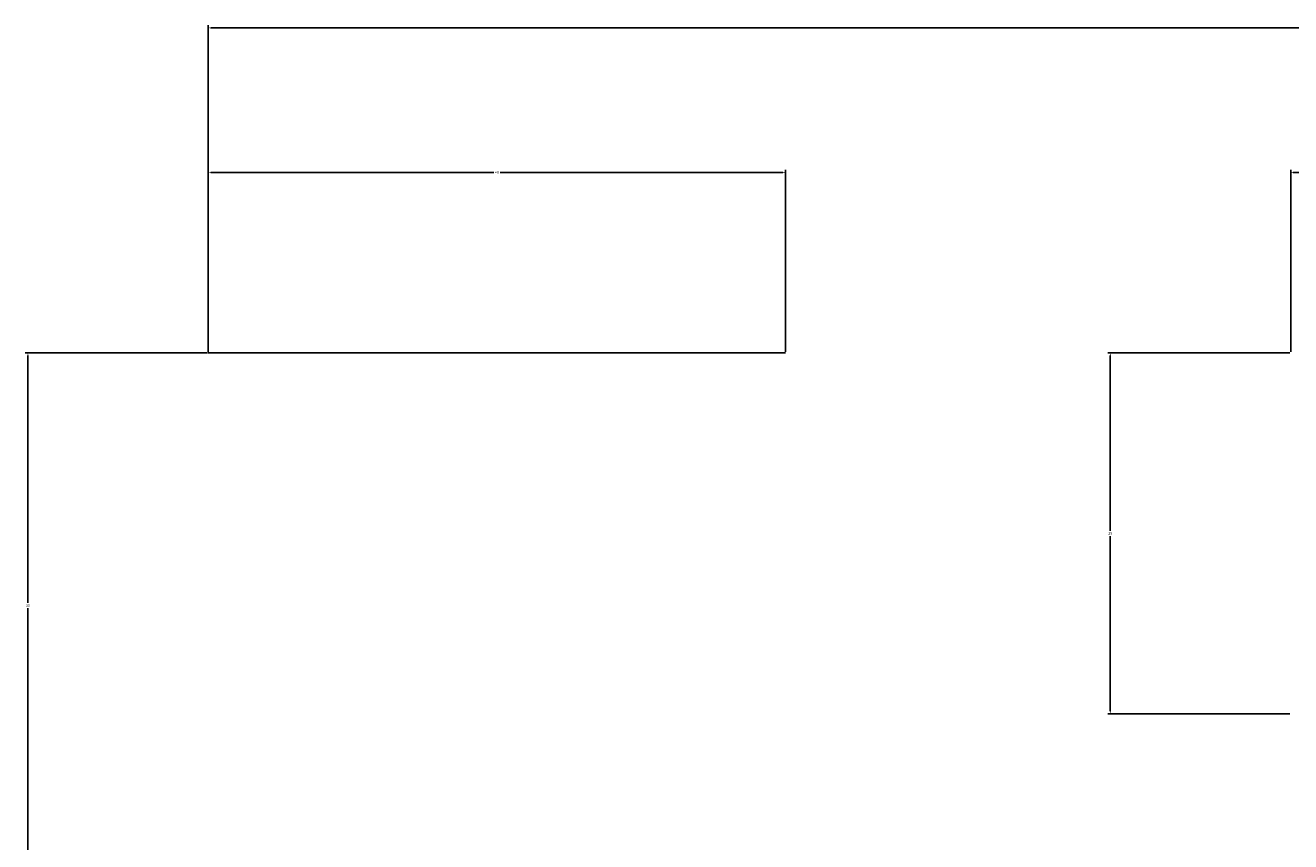
# Model space of a CAD drawing. Units: millimetres. Extents: x 135 to 361, y -58 to 58.
# Tile 2 of 5: x 135 to 223, y 1 to 58. Entities that reach past the tile are written whole.
import ezdxf

# ---------------------------------------------------------------- set-up
doc = ezdxf.new("R2010")
doc.units = ezdxf.units.MM
doc.layers.add('M-CONS', color=8, linetype='Continuous', lineweight=13)
doc.layers.add('M-DIMS', color=2, linetype='Continuous', lineweight=18)
doc.styles.get("Standard").update_dxf_attribs({"font": 'arial.ttf'})
doc.dimstyles.get("Standard").update_dxf_attribs({"dimtxt": 0.18, "dimasz": 0.18, "dimexe": 0.18, "dimexo": 0.0625, "dimgap": 0.09, "dimtad": 0, "dimtih": 1, "dimtoh": 1, "dimdec": 4, "dimzin": 0, "dimdsep": 46, "dimtxsty": 'Standard', "dimcen": 0.09, "dimadec": 0, "dimazin": 0, "dimtfac": 1, "dimtdec": 4, "dimtofl": 0, "dimtmove": 0, "dimatfit": 3, "dimfxl": 1, "dimtolj": 1, "dimtzin": 0, "dimarcsym": 0})

# ---------------------------------------------------------------- blocks, each defined once
blk = doc.blocks.new('*D1')
at = {"layer": 'Defpoints', "color": 0, "transparency": 16777216}
for p in [(347.813, 57.5), (347.813, 45), (147.813, 35)]:
    blk.add_point(p, dxfattribs=at)
at = {"layer": 'M-DIMS', "color": 0, "lineweight": -2, "transparency": 16777216}
for p, q in [((147.813, 35.062), (147.813, 57.68)), ((147.993, 57.5), (247.522, 57.5)), ((347.633, 57.5), (248.103, 57.5)), ((347.813, 45.062), (347.813, 57.68))]:
    blk.add_line(p, q, dxfattribs=at)
at = {"layer": 'M-DIMS', "color": 0, "transparency": 16777216}
for points in [[(147.993, 57.53), (147.993, 57.47), (147.813, 57.5)], [(347.633, 57.53), (347.633, 57.47), (347.813, 57.5)]]:
    blk.add_solid(points, dxfattribs=at)
at = {"layer": 'M-DIMS', "color": 0, "transparency": 16777216, "insert": (247.813, 57.5), "char_height": 0.18, "attachment_point": 5}
blk.add_mtext('\\A1;200', dxfattribs=at)
blk = doc.blocks.new('*D3')
at = {"layer": 'Defpoints', "color": 0, "transparency": 16777216}
for p in [(347.813, 47.5), (222.813, 35), (347.813, 35)]:
    blk.add_point(p, dxfattribs=at)
at = {"layer": 'M-DIMS', "color": 0, "lineweight": -2, "transparency": 16777216}
for p, q in [((222.813, 35.062), (222.813, 47.68)), ((222.993, 47.5), (285.031, 47.5)), ((347.633, 47.5), (285.594, 47.5)), ((347.813, 35.062), (347.813, 47.68))]:
    blk.add_line(p, q, dxfattribs=at)
at = {"layer": 'M-DIMS', "color": 0, "transparency": 16777216}
for points in [[(222.993, 47.53), (222.993, 47.47), (222.813, 47.5)], [(347.633, 47.53), (347.633, 47.47), (347.813, 47.5)]]:
    blk.add_solid(points, dxfattribs=at)
at = {"layer": 'M-DIMS', "color": 0, "transparency": 16777216, "insert": (285.313, 47.5), "char_height": 0.18, "attachment_point": 5}
blk.add_mtext('\\A1;125', dxfattribs=at)
blk = doc.blocks.new('*D4')
at = {"layer": 'Defpoints', "color": 0, "transparency": 16777216}
for p in [(210.313, 35), (222.813, 35), (222.813, 10)]:
    blk.add_point(p, dxfattribs=at)
at = {"layer": 'M-DIMS', "color": 0, "lineweight": -2, "transparency": 16777216}
for p, q in [((222.75, 35), (210.133, 35)), ((210.313, 34.82), (210.313, 22.682)), ((210.313, 10.18), (210.313, 22.318)), ((222.75, 10), (210.133, 10))]:
    blk.add_line(p, q, dxfattribs=at)
at = {"layer": 'M-DIMS', "color": 0, "transparency": 16777216}
for points in [[(210.283, 34.82), (210.343, 34.82), (210.313, 35)], [(210.283, 10.18), (210.343, 10.18), (210.313, 10)]]:
    blk.add_solid(points, dxfattribs=at)
at = {"layer": 'M-DIMS', "color": 0, "transparency": 16777216, "insert": (210.313, 22.5), "char_height": 0.18, "attachment_point": 5}
blk.add_mtext('\\A1;25', dxfattribs=at)
blk = doc.blocks.new('*D10')
at = {"layer": 'Defpoints', "color": 0, "transparency": 16777216}
for p in [(187.813, 47.5), (147.813, 35), (187.813, 35)]:
    blk.add_point(p, dxfattribs=at)
at = {"layer": 'M-DIMS', "color": 0, "lineweight": -2, "transparency": 16777216}
for p, q in [((147.813, 35.062), (147.813, 47.68)), ((147.993, 47.5), (167.59, 47.5)), ((187.633, 47.5), (168.035, 47.5)), ((187.813, 35.062), (187.813, 47.68))]:
    blk.add_line(p, q, dxfattribs=at)
at = {"layer": 'M-DIMS', "color": 0, "transparency": 16777216}
for points in [[(147.993, 47.53), (147.993, 47.47), (147.813, 47.5)], [(187.633, 47.53), (187.633, 47.47), (187.813, 47.5)]]:
    blk.add_solid(points, dxfattribs=at)
at = {"layer": 'M-DIMS', "color": 0, "transparency": 16777216, "insert": (167.813, 47.5), "char_height": 0.18, "attachment_point": 5}
blk.add_mtext('\\A1;40', dxfattribs=at)
blk = doc.blocks.new('*D11')
at = {"layer": 'Defpoints', "color": 0, "transparency": 16777216}
for p in [(135.313, 35), (147.813, 35), (147.813, 0)]:
    blk.add_point(p, dxfattribs=at)
at = {"layer": 'M-DIMS', "color": 0, "lineweight": -2, "transparency": 16777216}
for p, q in [((147.75, 35), (135.133, 35)), ((135.313, 34.82), (135.313, 17.682)), ((135.313, 0.18), (135.313, 17.318)), ((147.75, 0), (135.133, 0))]:
    blk.add_line(p, q, dxfattribs=at)
at = {"layer": 'M-DIMS', "color": 0, "transparency": 16777216}
for points in [[(135.283, 34.82), (135.343, 34.82), (135.313, 35)], [(135.283, 0.18), (135.343, 0.18), (135.313, 0)]]:
    blk.add_solid(points, dxfattribs=at)
at = {"layer": 'M-DIMS', "color": 0, "transparency": 16777216, "insert": (135.313, 17.5), "char_height": 0.18, "attachment_point": 5}
blk.add_mtext('\\A1;35', dxfattribs=at)

msp = doc.modelspace()

# ---------------------------------------------------------------- linework, layer by layer
at = {"layer": 'M-CONS', "extrusion": (0, -1, 0)}
msp.add_circle((167.813, 113.744, -35), 20, dxfattribs=at)

# ---------------------------------------------------------------- dimensions: what is measured, and where the dimension line sits
at = {"layer": 'M-DIMS'}
for base, p1, p2, picture, middle in [((347.813, 57.5), (147.813, 35), (347.813, 45), '*D1', (247.813, 57.5)), ((187.813, 47.5), (147.813, 35), (187.813, 35), '*D10', (167.813, 47.5)), ((347.813, 47.5), (222.813, 35), (347.813, 35), '*D3', (285.313, 47.5))]:
    dim = msp.add_linear_dim(base=base, p1=p1, p2=p2, dimstyle='Standard', override={"dimdec": 0, "dimlfac": 1, "dimrnd": 0, "dimzin": 0, "dimdsep": 46, "dimlunit": 2}, dxfattribs=at)
    dim.commit()
    dim.dimension.update_dxf_attribs({"geometry": picture, "text_midpoint": middle})
for base, p1, p2, picture, middle in [((135.313, 35), (147.813, 0), (147.813, 35), '*D11', (135.313, 17.5)), ((210.313, 35), (222.813, 10), (222.813, 35), '*D4', (210.313, 22.5))]:
    dim = msp.add_linear_dim(base=base, p1=p1, p2=p2, angle=90, dimstyle='Standard', override={"dimdec": 0, "dimlfac": 1, "dimrnd": 0, "dimzin": 0, "dimdsep": 46, "dimlunit": 2}, dxfattribs=at)
    dim.commit()
    dim.dimension.update_dxf_attribs({"geometry": picture, "text_midpoint": middle})

doc.saveas('drawing.dxf')
